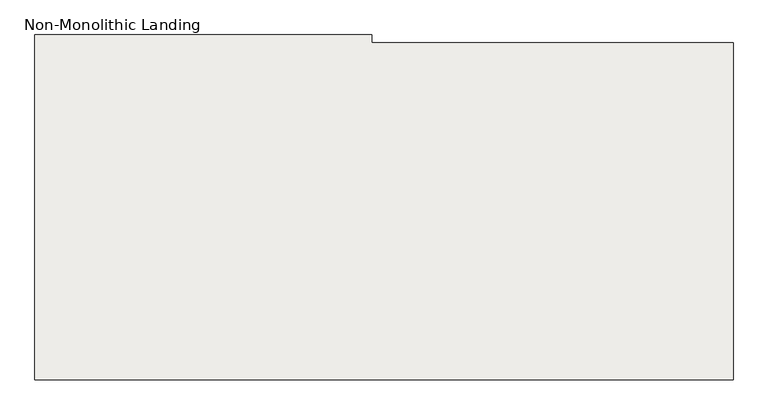
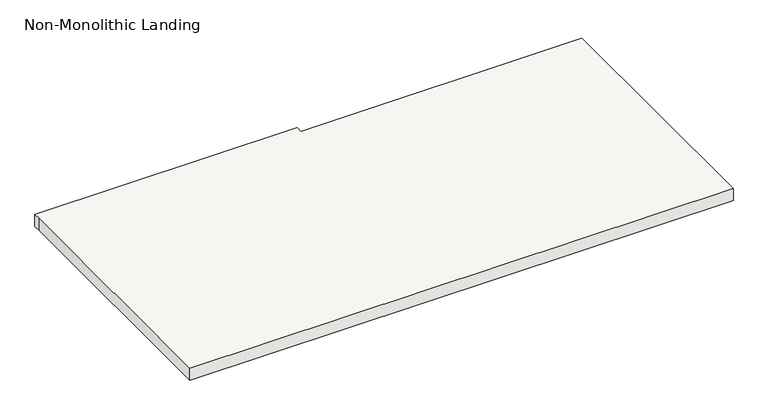
"""IFC4 building model written with IfcOpenShell, lengths in millimetres: slab geometry, Non-Monolithic Landing."""

from ifc_helpers import new_model, si_unit, origin, place, context, project, spatial, faceted_brep, source, transform, mapped, element, save


def non_monolithic_landing_af9dc4bc(model_context):
    return source(origin(), model_context, "Body", "Brep", [
        faceted_brep([(-5822.3581554, 4095.086641, 1733.55), (-5822.3581554, 4069.686641, 1708.15), (-6889.1581554, 4069.686641, 1708.15), (-6889.1581554, 4095.086641, 1733.55), (-6965.3581554, 4095.086641, 1752.6), (-6965.3581554, 4120.486641, 1752.6), (-8032.1581554, 4120.486641, 1752.6), (-8032.1581554, 4095.086641, 1752.6), (-8032.1581554, 3028.286641, 1752.6), (-5822.3581554, 3028.286641, 1752.6), (-5822.3581554, 4095.086641, 1752.6), (-6889.1581554, 4069.686641, 1701.8), (-5822.3581554, 4069.686641, 1701.8), (-5822.3581554, 3028.286641, 1701.8), (-8032.1581554, 3028.286641, 1701.8), (-8032.1581554, 4095.086641, 1701.8), (-8032.1581554, 4120.486641, 1701.8), (-6965.3581554, 4120.486641, 1701.8), (-6965.3581554, 4095.086641, 1701.8), (-6889.1581554, 4095.086641, 1701.8)], [[[0, 1, 2, 3]], [[4, 5, 6, 7, 8, 9, 10]], [[11, 12, 13, 14, 15, 16, 17, 18, 19]], [[12, 11, 2, 1]], [[11, 19, 3, 2]], [[4, 10, 0, 3, 19, 18]], [[5, 4, 18, 17]], [[6, 5, 17, 16]], [[7, 6, 16, 15]], [[8, 7, 15, 14]], [[9, 8, 14, 13]], [[10, 9, 13, 12, 1, 0]]]),
    ])


if __name__ == "__main__":
    model = new_model("IFC4")
    model_context = context("Model", 3, world=origin())
    ifc_project = project(units=[si_unit("LENGTHUNIT", "METRE", prefix="MILLI")], contexts=[model_context])
    site = spatial("IfcSite", under=ifc_project)
    building = spatial("IfcBuilding", under=site)
    placement = place(None, origin())
    non_monolithic_landing_shape = non_monolithic_landing_af9dc4bc(model_context)
    element("IfcSlab", 1, ObjectType="Non-Monolithic Landing", at=placement, inside=building, context=model_context, shape_type="MappedRepresentation", body=[
        mapped(non_monolithic_landing_shape, transform((0.0, 0.0, 0.0), x_axis=(1.0, 0.0, 0.0), y_axis=(0.0, 1.0, 0.0), z_axis=(0.0, 0.0, 1.0))),
    ])
    save(model, "model.ifc")
